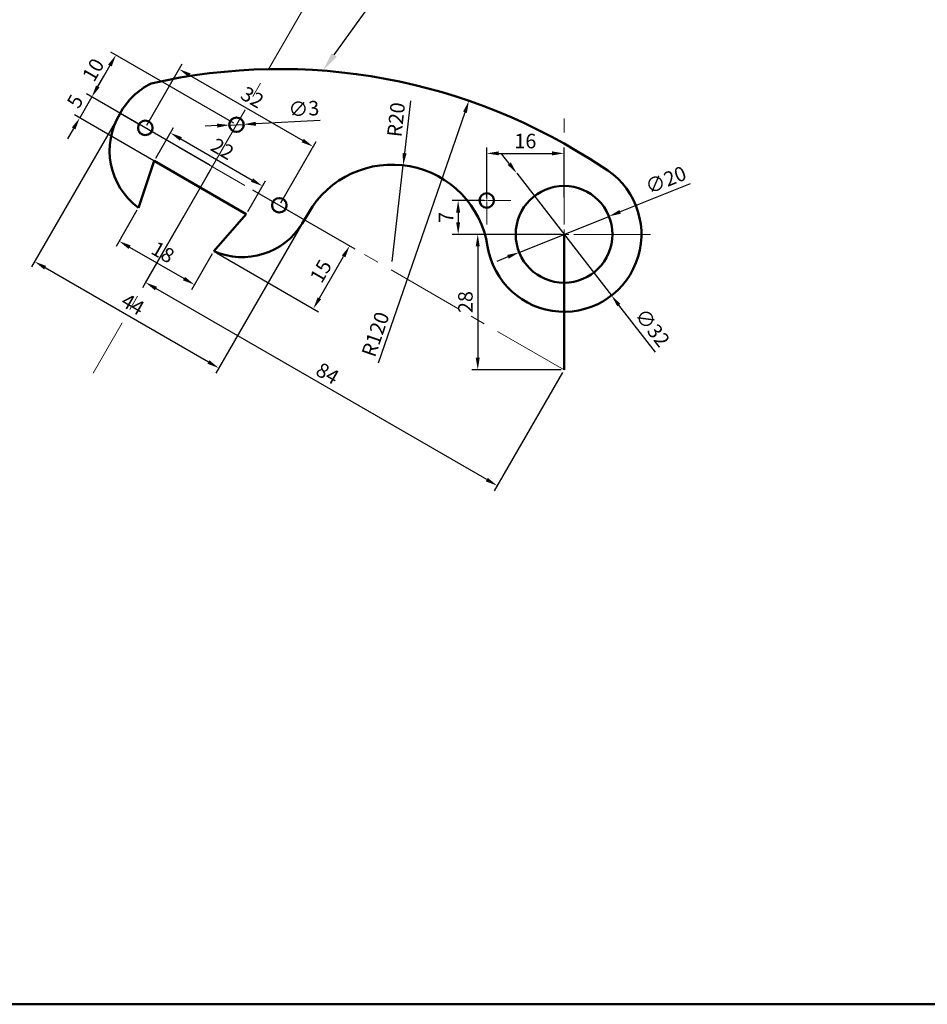
# Model space of a CAD drawing. Units: millimetres. Extents: x 77 to 718, y -35 to 313.
# Tile 2 of 7: x 191 to 379, y -35 to 169. Entities that reach past the tile are written whole.
import ezdxf
from ezdxf import colors
from ezdxf.entities.mleader import LeaderData, LeaderLine
from ezdxf.math import Vec2, Vec3

# ---------------------------------------------------------------- set-up
doc = ezdxf.new("R2010")
doc.units = ezdxf.units.MM
doc.header["$LTSCALE"] = 0.5
doc.linetypes.add('CENTER', pattern=[50.8, 31.75, -6.35, 6.35, -6.35])
for name, color, linetype, lineweight in [('M-CNTR', 1, 'CENTER', 18), ('M-DIMS', 2, 'Continuous', 25), ('M-OUTL', 7, 'Continuous', 50), ('M-TEXT', 3, 'Continuous', 25)]:
    doc.layers.add(name, color=color, linetype=linetype, lineweight=lineweight)
doc.styles.get("Standard").update_dxf_attribs({"font": 'arial.ttf'})
doc.dimstyles.new('ISO-25', dxfattribs={"dimtxt": 3, "dimasz": 2.5, "dimexe": 1.25, "dimexo": 0.625, "dimtad": 1, "dimtxsty": 'Standard', "dimcen": 2.5, "dimadec": 0, "dimazin": 0, "dimtfac": 1, "dimtmove": 0, "dimatfit": 3, "dimfxl": 1, "dimarcsym": 0})

# ---------------------------------------------------------------- blocks, each defined once
blk = doc.blocks.new('*U49')
at = {"layer": 'M-CNTR', "color": 0, "transparency": 16777216}
for p, q in [((0, 2), (0, 23.94)), ((-21.91, 0), (-2, 0)), ((2, 0), (21.02, 0)), ((0, -13.5), (0, -2))]:
    blk.add_line(p, q, dxfattribs=at)
at = {"layer": 'M-CNTR', "color": 0, "linetype": 'Continuous', "transparency": 16777216}
for p, q in [((-1, 0), (1, 0)), ((0, -1), (0, 1))]:
    blk.add_line(p, q, dxfattribs=at)
blk = doc.blocks.new('*D50')
at = {"layer": 'Defpoints', "color": 0, "transparency": 16777216}
for p in [(216.04, 129.74), (231.63, 120.74), (227.64, 113.83)]:
    blk.add_point(p, dxfattribs=at)
at = {"layer": 'M-DIMS', "color": 0, "lineweight": -2, "transparency": 16777216}
for p, q in [((215.73, 129.2), (211.43, 121.75)), ((214.22, 121.58), (225.48, 115.08)), ((231.32, 120.2), (227.02, 112.75))]:
    blk.add_line(p, q, dxfattribs=at)
at = {"layer": 'M-DIMS', "color": 0, "transparency": 16777216}
for points in [[(214.43, 121.94), (214.01, 121.22), (212.06, 122.83)], [(225.69, 115.44), (225.27, 114.72), (227.64, 113.83)]]:
    blk.add_solid(points, dxfattribs=at)
at = {"layer": 'M-DIMS', "color": 0, "transparency": 16777216, "insert": (220.93, 120.2), "char_height": 3, "attachment_point": 5, "rotation": 330}
blk.add_mtext('18', dxfattribs=at)
blk = doc.blocks.new('*D51')
at = {"layer": 'Defpoints', "color": 0, "transparency": 16777216}
for p in [(212.28, 149.23), (250.39, 127.23), (194.6, 118.59)]:
    blk.add_point(p, dxfattribs=at)
at = {"layer": 'M-DIMS', "color": 0, "lineweight": -2, "transparency": 16777216}
for p, q in [((211.97, 148.69), (193.97, 117.51)), ((250.08, 126.69), (232.08, 95.51)), ((230.54, 97.84), (196.76, 117.34))]:
    blk.add_line(p, q, dxfattribs=at)
at = {"layer": 'M-DIMS', "color": 0, "transparency": 16777216}
for points in [[(196.97, 117.7), (196.55, 116.98), (194.6, 118.59)], [(230.74, 98.2), (230.33, 97.48), (232.7, 96.59)]]:
    blk.add_solid(points, dxfattribs=at)
at = {"layer": 'M-DIMS', "color": 0, "transparency": 16777216, "insert": (214.71, 109.43), "char_height": 3, "attachment_point": 5, "rotation": 330}
blk.add_mtext('44', dxfattribs=at)
blk = doc.blocks.new('*D52')
at = {"layer": 'Defpoints', "color": 0, "transparency": 16777216}
for p in [(217.48, 146.23), (252.19, 142.35), (245.19, 130.23)]:
    blk.add_point(p, dxfattribs=at)
at = {"layer": 'M-DIMS', "color": 0, "lineweight": -2, "transparency": 16777216}
for p, q in [((217.79, 146.77), (225.11, 159.44)), ((226.65, 157.1), (250.03, 143.6)), ((245.51, 130.77), (252.82, 143.44))]:
    blk.add_line(p, q, dxfattribs=at)
at = {"layer": 'M-DIMS', "color": 0, "transparency": 16777216}
for points in [[(226.86, 157.47), (226.44, 156.74), (224.48, 158.35)], [(250.24, 143.97), (249.82, 143.24), (252.19, 142.35)]]:
    blk.add_solid(points, dxfattribs=at)
at = {"layer": 'M-DIMS', "color": 0, "transparency": 16777216, "insert": (239.42, 152.22), "char_height": 3, "attachment_point": 5, "rotation": 330}
blk.add_mtext('32', dxfattribs=at)
blk = doc.blocks.new('*D53')
at = {"layer": 'Defpoints', "color": 0, "transparency": 16777216}
for p in [(239.13, 133.73), (231.63, 120.74), (259.73, 121.84)]:
    blk.add_point(p, dxfattribs=at)
at = {"layer": 'M-DIMS', "color": 0, "lineweight": -2, "transparency": 16777216}
for p, q in [((239.67, 133.42), (260.81, 121.21)), ((232.17, 120.43), (253.31, 108.22)), ((253.48, 111.01), (258.48, 119.67))]:
    blk.add_line(p, q, dxfattribs=at)
at = {"layer": 'M-DIMS', "color": 0, "transparency": 16777216}
for points in [[(258.12, 119.88), (258.84, 119.46), (259.73, 121.84)], [(253.12, 111.22), (253.84, 110.8), (252.23, 108.85)]]:
    blk.add_solid(points, dxfattribs=at)
at = {"layer": 'M-DIMS', "color": 0, "transparency": 16777216, "insert": (254.11, 116.42), "char_height": 3, "attachment_point": 5, "rotation": 60}
blk.add_mtext('15', dxfattribs=at)
blk = doc.blocks.new('*D54')
at = {"layer": 'Defpoints', "color": 0, "transparency": 16777216}
for p in [(231.34, 138.23), (217.51, 114.29), (304.08, 96.23)]:
    blk.add_point(p, dxfattribs=at)
at = {"layer": 'M-DIMS', "color": 0, "lineweight": -2, "transparency": 16777216}
for p, q in [((231.02, 137.69), (216.89, 113.2)), ((288.09, 73.54), (219.68, 113.04)), ((303.77, 95.69), (289.63, 71.2))]:
    blk.add_line(p, q, dxfattribs=at)
at = {"layer": 'M-DIMS', "color": 0, "transparency": 16777216}
for points in [[(219.89, 113.4), (219.47, 112.67), (217.51, 114.29)], [(288.3, 73.9), (287.89, 73.17), (290.26, 72.29)]]:
    blk.add_solid(points, dxfattribs=at)
at = {"layer": 'M-DIMS', "color": 0, "transparency": 16777216, "insert": (254.97, 95.15), "char_height": 3, "attachment_point": 5, "rotation": 330}
blk.add_mtext('84', dxfattribs=at)
blk = doc.blocks.new('*U55')
at = {"layer": 'M-CNTR', "color": 0, "transparency": 16777216}
for p, q in [((0, 0.3), (0, 5)), ((-5, 0), (-0.3, 0)), ((0.3, 0), (5, 0)), ((0, -5), (0, -0.3))]:
    blk.add_line(p, q, dxfattribs=at)
at = {"layer": 'M-CNTR', "color": 0, "linetype": 'Continuous', "transparency": 16777216}
for p, q in [((-0.15, 0), (0.15, 0)), ((0, -0.15), (0, 0.15))]:
    blk.add_line(p, q, dxfattribs=at)
blk = doc.blocks.new('*D56')
at = {"layer": 'Defpoints', "color": 0, "transparency": 16777216}
for p in [(294.28, 136.87), (313.89, 111.58)]:
    blk.add_point(p, dxfattribs=at)
at = {"layer": 'M-DIMS', "color": 0, "lineweight": -2, "transparency": 16777216}
for p, q in [((292.75, 138.85), (291.22, 140.82)), ((294.28, 136.87), (313.89, 111.58)), ((322.98, 99.86), (315.42, 109.61))]:
    blk.add_line(p, q, dxfattribs=at)
at = {"layer": 'M-DIMS', "color": 0, "transparency": 16777216}
for points in [[(293.08, 139.1), (292.42, 138.59), (294.28, 136.87)], [(315.75, 109.86), (315.09, 109.35), (313.89, 111.58)]]:
    blk.add_solid(points, dxfattribs=at)
at = {"layer": 'M-DIMS', "color": 0, "transparency": 16777216, "insert": (322.06, 104.7), "char_height": 3, "attachment_point": 5, "rotation": 307.7882}
blk.add_mtext('∅32', dxfattribs=at)
blk = doc.blocks.new('*D57')
at = {"layer": 'Defpoints', "color": 0, "transparency": 16777216}
for p in [(313.37, 127.95), (294.8, 120.51)]:
    blk.add_point(p, dxfattribs=at)
at = {"layer": 'M-DIMS', "color": 0, "lineweight": -2, "transparency": 16777216}
for p, q in [((330.18, 134.68), (315.69, 128.88)), ((294.8, 120.51), (313.37, 127.95)), ((292.48, 119.58), (290.16, 118.65))]:
    blk.add_line(p, q, dxfattribs=at)
at = {"layer": 'M-DIMS', "color": 0, "transparency": 16777216}
for points in [[(315.53, 129.26), (315.84, 128.49), (313.37, 127.95)], [(292.32, 119.97), (292.63, 119.19), (294.8, 120.51)]]:
    blk.add_solid(points, dxfattribs=at)
at = {"layer": 'M-DIMS', "color": 0, "transparency": 16777216, "insert": (325.26, 135.12), "char_height": 3, "attachment_point": 5, "rotation": 21.8253}
blk.add_mtext('∅20', dxfattribs=at)
blk = doc.blocks.new('*D58')
at = {"layer": 'Defpoints', "color": 0, "transparency": 16777216}
for p in [(206.41, 152.62), (236.34, 146.89), (231.34, 138.23)]:
    blk.add_point(p, dxfattribs=at)
at = {"layer": 'M-DIMS', "color": 0, "lineweight": -2, "transparency": 16777216}
for p, q in [((235.8, 147.2), (210.32, 161.91)), ((210.16, 159.12), (207.66, 154.79)), ((230.8, 138.54), (205.32, 153.25))]:
    blk.add_line(p, q, dxfattribs=at)
at = {"layer": 'M-DIMS', "color": 0, "transparency": 16777216}
for points in [[(209.79, 159.33), (210.52, 158.91), (211.41, 161.28)], [(207.29, 155), (208.02, 154.58), (206.41, 152.62)]]:
    blk.add_solid(points, dxfattribs=at)
at = {"layer": 'M-DIMS', "color": 0, "transparency": 16777216, "insert": (207.04, 158.03), "char_height": 3, "attachment_point": 5, "rotation": 60}
blk.add_mtext('10', dxfattribs=at)
blk = doc.blocks.new('*D59')
at = {"layer": 'Defpoints', "color": 0, "transparency": 16777216}
for p in [(203.91, 148.29), (231.34, 138.23), (228.84, 133.9)]:
    blk.add_point(p, dxfattribs=at)
at = {"layer": 'M-DIMS', "color": 0, "lineweight": -2, "transparency": 16777216}
for p, q in [((207.66, 154.79), (208.91, 156.95)), ((206.41, 152.62), (203.91, 148.29)), ((230.8, 138.54), (205.32, 153.25)), ((228.3, 134.21), (202.82, 148.92)), ((202.66, 146.13), (201.41, 143.96))]:
    blk.add_line(p, q, dxfattribs=at)
at = {"layer": 'M-DIMS', "color": 0, "transparency": 16777216}
for points in [[(207.29, 155), (208.02, 154.58), (206.41, 152.62)], [(202.29, 146.34), (203.02, 145.92), (203.91, 148.29)]]:
    blk.add_solid(points, dxfattribs=at)
at = {"layer": 'M-DIMS', "color": 0, "transparency": 16777216, "insert": (203.29, 151.53), "char_height": 3, "attachment_point": 5, "rotation": 60}
blk.add_mtext('5', dxfattribs=at)
blk = doc.blocks.new('*D60')
at = {"layer": 'Defpoints', "color": 0, "transparency": 16777216}
for p in [(304.08, 140.96), (288.08, 131.23), (304.08, 131.23)]:
    blk.add_point(p, dxfattribs=at)
at = {"layer": 'M-DIMS', "color": 0, "lineweight": -2, "transparency": 16777216}
for p, q in [((288.08, 131.85), (288.08, 142.21)), ((290.58, 140.96), (301.58, 140.96)), ((304.08, 131.85), (304.08, 142.21))]:
    blk.add_line(p, q, dxfattribs=at)
at = {"layer": 'M-DIMS', "color": 0, "transparency": 16777216}
for points in [[(290.58, 141.38), (290.58, 140.55), (288.08, 140.96)], [(301.58, 141.38), (301.58, 140.55), (304.08, 140.96)]]:
    blk.add_solid(points, dxfattribs=at)
at = {"layer": 'M-DIMS', "color": 0, "transparency": 16777216, "insert": (296.08, 143.12), "char_height": 3, "attachment_point": 5}
blk.add_mtext('16', dxfattribs=at)
blk = doc.blocks.new('*D61')
at = {"layer": 'Defpoints', "color": 0, "transparency": 16777216}
for p in [(288.08, 131.23), (282.18, 124.23), (288.08, 124.23)]:
    blk.add_point(p, dxfattribs=at)
at = {"layer": 'M-DIMS', "color": 0, "lineweight": -2, "transparency": 16777216}
for p, q in [((287.46, 131.23), (280.93, 131.23)), ((282.18, 128.73), (282.18, 126.73)), ((287.46, 124.23), (280.93, 124.23))]:
    blk.add_line(p, q, dxfattribs=at)
at = {"layer": 'M-DIMS', "color": 0, "transparency": 16777216}
for points in [[(281.76, 128.73), (282.59, 128.73), (282.18, 131.23)], [(281.76, 126.73), (282.59, 126.73), (282.18, 124.23)]]:
    blk.add_solid(points, dxfattribs=at)
at = {"layer": 'M-DIMS', "color": 0, "transparency": 16777216, "insert": (280.05, 127.73), "char_height": 3, "attachment_point": 5, "rotation": 90}
blk.add_mtext('7', dxfattribs=at)
blk = doc.blocks.new('*D62')
at = {"layer": 'Defpoints', "color": 0, "transparency": 16777216}
for p in [(304.08, 124.23), (286.23, 96.23), (304.08, 96.23)]:
    blk.add_point(p, dxfattribs=at)
at = {"layer": 'M-DIMS', "color": 0, "lineweight": -2, "transparency": 16777216}
for p, q in [((303.46, 124.23), (284.98, 124.23)), ((286.23, 121.73), (286.23, 98.73)), ((303.46, 96.23), (284.98, 96.23))]:
    blk.add_line(p, q, dxfattribs=at)
at = {"layer": 'M-DIMS', "color": 0, "transparency": 16777216}
for points in [[(285.81, 121.73), (286.64, 121.73), (286.23, 124.23)], [(285.81, 98.73), (286.64, 98.73), (286.23, 96.23)]]:
    blk.add_solid(points, dxfattribs=at)
at = {"layer": 'M-DIMS', "color": 0, "transparency": 16777216, "insert": (284.07, 110.23), "char_height": 3, "attachment_point": 5, "rotation": 90}
blk.add_mtext('28', dxfattribs=at)
blk = doc.blocks.new('*D63')
at = {"layer": 'Defpoints', "color": 0, "transparency": 16777216}
for p in [(219.31, 139.4), (241.71, 134.2), (238.36, 128.4)]:
    blk.add_point(p, dxfattribs=at)
at = {"layer": 'M-DIMS', "color": 0, "lineweight": -2, "transparency": 16777216}
for p, q in [((219.62, 139.94), (223.29, 146.28)), ((224.83, 143.95), (239.55, 135.45)), ((238.68, 128.94), (242.34, 135.28))]:
    blk.add_line(p, q, dxfattribs=at)
at = {"layer": 'M-DIMS', "color": 0, "transparency": 16777216}
for points in [[(225.04, 144.31), (224.62, 143.59), (222.66, 145.2)], [(239.76, 135.81), (239.34, 135.09), (241.71, 134.2)]]:
    blk.add_solid(points, dxfattribs=at)
at = {"layer": 'M-DIMS', "color": 0, "transparency": 16777216, "insert": (233.25, 141.55), "char_height": 3, "attachment_point": 5, "rotation": 330}
blk.add_mtext('22', dxfattribs=at)
blk = doc.blocks.new('*D64')
at = {"layer": 'Defpoints', "color": 0, "transparency": 16777216}
for p in [(234.84, 146.82), (237.84, 146.96)]:
    blk.add_point(p, dxfattribs=at)
at = {"layer": 'M-DIMS', "color": 0, "lineweight": -2, "transparency": 16777216}
for p, q in [((232.34, 146.69), (229.85, 146.57)), ((234.84, 146.82), (237.84, 146.96)), ((253.64, 147.74), (240.33, 147.09))]:
    blk.add_line(p, q, dxfattribs=at)
at = {"layer": 'M-DIMS', "color": 0, "transparency": 16777216}
for points in [[(232.32, 147.11), (232.36, 146.28), (234.84, 146.82)], [(240.31, 147.5), (240.35, 146.67), (237.84, 146.96)]]:
    blk.add_solid(points, dxfattribs=at)
at = {"layer": 'M-DIMS', "color": 0, "transparency": 16777216, "insert": (250.29, 149.82), "char_height": 3, "attachment_point": 5, "rotation": 2.8277}
blk.add_mtext('∅3', dxfattribs=at)
blk = doc.blocks.new('*D65')
at = {"layer": 'Defpoints', "color": 0, "transparency": 16777216}
for p in [(270.81, 138.5), (268.52, 118.63)]:
    blk.add_point(p, dxfattribs=at)
at = {"layer": 'M-DIMS', "color": 0, "lineweight": -2, "transparency": 16777216}
for p, q in [((272.35, 151.82), (271.1, 140.98)), ((268.52, 118.63), (270.81, 138.5))]:
    blk.add_line(p, q, dxfattribs=at)
at = {"layer": 'M-DIMS', "color": 0, "transparency": 16777216}
blk.add_solid([(270.68, 141.03), (271.51, 140.94), (270.81, 138.5)], dxfattribs=at)
at = {"layer": 'M-DIMS', "color": 0, "transparency": 16777216, "insert": (269.72, 147.89), "char_height": 3, "attachment_point": 5, "rotation": 83.4212}
blk.add_mtext('R20', dxfattribs=at)
blk = doc.blocks.new('*D66')
at = {"layer": 'Defpoints', "color": 0, "transparency": 16777216}
for p in [(284.41, 151.83), (245.27, 38.39)]:
    blk.add_point(p, dxfattribs=at)
at = {"layer": 'M-DIMS', "color": 0, "lineweight": -2, "transparency": 16777216}
blk.add_line((265.73, 97.68), (283.6, 149.47), dxfattribs=at)
at = {"layer": 'M-DIMS', "color": 0, "transparency": 16777216}
blk.add_solid([(283.2, 149.6), (283.99, 149.33), (284.41, 151.83)], dxfattribs=at)
at = {"layer": 'M-DIMS', "color": 0, "transparency": 16777216, "insert": (265.44, 103.45), "char_height": 3, "attachment_point": 5, "rotation": 70.9639}
blk.add_mtext('R120', dxfattribs=at)

msp = doc.modelspace()

# ---------------------------------------------------------------- linework, layer by layer
at = {"layer": 'M-CNTR'}
for p, q in [((250.801, 171.941), (206.682, 95.525)), ((304.083, 96.229), (212.285, 149.229))]:
    msp.add_line(p, q, dxfattribs=at)
at = {"layer": 'M-OUTL'}
for p, q in [((216.043, 129.738), (219.311, 139.399)), ((219.311, 139.399), (238.364, 128.399)), ((231.631, 120.738), (238.364, 128.399)), ((251.2, 128.633), (249.952, 126.47)), ((304.083, 124.229), (304.083, 96.229))]:
    msp.add_line(p, q, dxfattribs=at)
at = {"layer": 'M-OUTL', "ltscale": 0.5}
msp.add_lwpolyline([(77.418, 312.912), (718.012, 312.912), (718.012, -34.898), (77.418, -34.898)], close=True, dxfattribs=at)
at = {"layer": 'M-OUTL'}
for centre, radius in [((217.481, 146.229), 1.5), ((236.337, 146.889), 1.5), ((288.083, 131.229), 1.5), ((304.083, 124.229), 10), ((245.194, 130.229), 1.5)]:
    msp.add_circle(centre, radius, dxfattribs=at)
for centre, radius, start, end in [((245.272, 38.393), 120, 56.23568, 102.80979), ((225.19, 142.284), 14.655, 116.43382, 151.71188), ((224.752, 141.525), 14.655, 148.28812, 233.54065), ((268.521, 118.633), 20, 8.94244, 150), ((304.083, 124.229), 16, 188.94244, 60.4886), ((237.485, 134.174), 14.655, 246.45935, 328.28812)]:
    msp.add_arc(centre, radius, start, end, dxfattribs=at)

# ---------------------------------------------------------------- block references
at = {"layer": 'M-CNTR'}
for name, p in [('*U49', (304.083, 124.229)), ('*U55', (288.083, 131.229))]:
    msp.add_blockref(name, p, dxfattribs=at)

# ---------------------------------------------------------------- dimensions: what is measured, and where the dimension line sits
at = {"layer": 'M-DIMS'}
for p1, p2, distance, picture, middle in [((236.337, 146.889), (231.337, 138.229), -28.789, '*D58', (207.038, 158.032)), ((217.481, 146.229), (245.194, 130.229), 14.002, '*D52', (239.417, 152.223)), ((231.337, 138.229), (228.837, 133.899), -28.789, '*D59', (203.293, 151.533)), ((250.39, 127.229), (212.285, 149.229), 35.378, '*D51', (214.711, 109.431)), ((219.311, 139.399), (238.364, 128.399), 6.702, '*D63', (233.254, 141.548)), ((304.083, 96.229), (231.337, 138.229), 27.647, '*D54', (254.965, 95.153)), ((231.631, 120.738), (239.131, 133.729), -23.782, '*D53', (254.11, 116.421)), ((216.043, 129.738), (231.631, 120.738), -7.975, '*D50', (220.928, 120.2))]:
    dim = msp.add_aligned_dim(p1=p1, p2=p2, distance=distance, dimstyle='ISO-25', override={"dimclrd": 0, "dimclre": 0, "dimclrt": 0}, dxfattribs=at)
    dim.commit()
    dim.dimension.update_dxf_attribs({"geometry": picture, "text_midpoint": middle})
for p1, p2, picture, middle in [((234.839, 146.815), (237.835, 146.963), '*D64', (250.402, 147.584)), ((294.279, 136.873), (313.887, 111.584), '*D56', (320.287, 103.331)), ((294.8, 120.511), (313.367, 127.947), '*D57', (326.093, 133.043))]:
    dim = msp.add_diameter_dim_2p(p1=p1, p2=p2, dimstyle='ISO-25', override={"dimclrd": 0, "dimclre": 0, "dimclrt": 0}, dxfattribs=at)
    dim.commit()
    dim.dimension.update_dxf_attribs({"geometry": picture, "text_midpoint": middle, "dimtype": 163})
dim = msp.add_radius_dim(center=(245.272, 38.393), mpoint=(284.411, 151.831), dimstyle='ISO-25', override={"dimclrd": 0, "dimclre": 0, "dimclrt": 0}, dxfattribs=at)
dim.commit()
dim.dimension.update_dxf_attribs({"geometry": '*D66', "text_midpoint": (267.477, 102.751), "dimtype": 164})
dim = msp.add_radius_dim(center=(268.521, 118.633), mpoint=(270.812, 138.501), dimstyle='ISO-25', override={"dimclrd": 0, "dimclre": 0, "dimclrt": 0}, dxfattribs=at)
dim.commit()
dim.dimension.update_dxf_attribs({"geometry": '*D65', "text_midpoint": (269.724, 147.892)})
dim = msp.add_linear_dim(base=(304.083, 140.963), p1=(288.083, 131.229), p2=(304.083, 131.229), dimstyle='ISO-25', override={"dimclrd": 0, "dimclre": 0, "dimclrt": 0}, dxfattribs=at)
dim.commit()
dim.dimension.update_dxf_attribs({"geometry": '*D60', "text_midpoint": (296.083, 143.12)})
for base, p1, p2, picture, middle in [((282.175, 124.229), (288.083, 131.229), (288.083, 124.229), '*D61', (280.05, 127.729)), ((286.228, 96.229), (304.083, 124.229), (304.083, 96.229), '*D62', (284.072, 110.229))]:
    dim = msp.add_linear_dim(base=base, p1=p1, p2=p2, angle=90, dimstyle='ISO-25', override={"dimclrd": 0, "dimclre": 0, "dimclrt": 0}, dxfattribs=at)
    dim.commit()
    dim.dimension.update_dxf_attribs({"geometry": picture, "text_midpoint": middle})

# ---------------------------------------------------------------- leaders
at = {"layer": 'M-TEXT'}
ml = msp.add_multileader_mtext('Standard', dxfattribs=at)
ml.set_content('1', color=256)
ml.set_leader_properties()
ml.build(insert=Vec2(0, 0))
ctx = ml.context
ctx.base_point, ctx.char_height, ctx.plane_origin = Vec3(274.991, 175.877), 8, Vec3(254.229, 158.058)
notes = []
notes.append((ctx, [(0, (1, 1, 0), (266.991, 175.877), (1, 0), 8, [(0, [(254.229, 158.058)], 0, [])])]))
ctx.mtext.insert, ctx.mtext.flow_direction = Vec3(276.991, 179.877), 5
for ctx, leaders in notes:
    for number, flags, end, landing, length, lines in leaders:
        leader = LeaderData()
        leader.index, (leader.has_last_leader_line, leader.has_dogleg_vector, leader.attachment_direction) = number, flags
        leader.last_leader_point, leader.dogleg_vector, leader.dogleg_length = Vec3(end), Vec3(landing), length
        for number, points, colour, breaks in lines:
            line = LeaderLine()
            line.index, line.vertices, line.color, line.breaks = number, Vec3.list(points), colors.encode_raw_color(colour), breaks
            leader.lines.append(line)
        ctx.leaders.append(leader)

doc.saveas('drawing.dxf')
